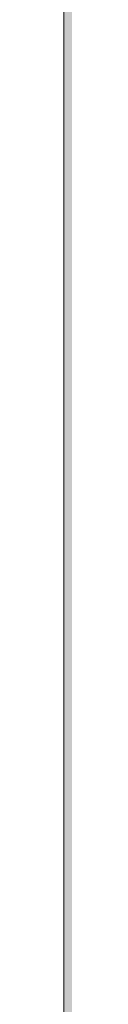
# Model space of a CAD drawing. Units: inches. Extents: x 459864 to 460310, y 324185 to 324787.
# Tile 34 of 112: x 460077.909 to 460077.909, y 324235.812 to 324241.994. Entities that reach past the tile are written whole.
import ezdxf

# ---------------------------------------------------------------- set-up
doc = ezdxf.new("R2010")
doc.units = ezdxf.units.IN
for name, color, linetype, lineweight in [('A-ANNO-DIMS', 2, 'Continuous', 18), ('L-HRDS', 9, 'Continuous', 18), ('L-SITE-PATT', 252, 'Continuous', 13)]:
    doc.layers.add(name, color=color, linetype=linetype, lineweight=lineweight)
doc.styles.get("Standard").update_dxf_attribs({"font": 'arial.ttf'})
doc.dimstyles.new('ISO-25', dxfattribs={"dimtxt": 6, "dimasz": 2.5, "dimexe": 1.25, "dimexo": 0.625, "dimtad": 1, "dimdec": 1, "dimlunit": 3, "dimtxsty": 'Standard', "dimcen": 2.5, "dimadec": 0, "dimazin": 0, "dimtfac": 1, "dimtdec": 1, "dimtmove": 0, "dimatfit": 3, "dimfxl": 1, "dimarcsym": 0})

# ---------------------------------------------------------------- blocks, each defined once
blk = doc.blocks.new('*D36')
at = {"layer": 'A-ANNO-DIMS', "color": 0, "lineweight": -2, "transparency": 16777216}
for p, q in [((460063.8613, 324228.4828), (460063.8613, 324226.0557)), ((460075.8757, 324228.4828), (460075.8757, 324226.0557)), ((460066.3613, 324227.3057), (460073.3757, 324227.3057)), ((460075.8757, 324227.3057), (460126.0214, 324227.3057))]:
    blk.add_line(p, q, dxfattribs=at)
at = {"layer": 'A-ANNO-DIMS', "color": 0, "transparency": 16777216}
for points in [[(460066.3613, 324227.7223), (460066.3613, 324226.889), (460063.8613, 324227.3057)], [(460073.3757, 324227.7223), (460073.3757, 324226.889), (460075.8757, 324227.3057)]]:
    blk.add_solid(points, dxfattribs=at)
at = {"layer": 'Defpoints', "color": 0, "transparency": 16777216}
for p in [(460063.8613, 324229.1078), (460075.8757, 324229.1078), (460075.8757, 324227.3057)]:
    blk.add_point(p, dxfattribs=at)
at = {"layer": 'A-ANNO-DIMS', "color": 0, "transparency": 16777216, "insert": (460102.1986, 324230.9941), "char_height": 6, "attachment_point": 5}
blk.add_mtext('PAVER 1\'-0"', dxfattribs=at)

msp = doc.modelspace()

# ---------------------------------------------------------------- hatches: boundary and pattern name
at = {"layer": 'L-SITE-PATT'}
h = msp.add_hatch(dxfattribs=at)
h.set_pattern_fill('DOTS', color=256)
h.paths.add_polyline_path([(460269.8036, 324283.4832), (460247.1149, 324283.4832), (460121.9293, 324283.4832), (460121.9293, 324252.473), (460117.4293, 324252.473), (460110.1236, 324252.473), (460110.1236, 324243.2865), (460080.8295, 324243.2865), (460080.8295, 324252.473), (460061.1149, 324252.473), (460061.1149, 324251.8824), (460077.9089, 324251.8824), (460077.9089, 324199.4832), (460080.8295, 324199.4832), (460080.8295, 324207.5532), (460110.1236, 324207.5532), (460110.1236, 324199.4832), (460110.8133, 324199.4832), (460262.1149, 324199.4832), (460269.8036, 324199.4832)], flags=17)
edge = h.paths.add_edge_path(flags=0)
edge.add_ellipse((460222.5903, 324263.8132), major_axis=(-8.4853, 8.4853), ratio=1, start_angle=405, end_angle=495, ccw=False)
edge.add_line((460214.8209, 324254.6599), (460214.8316, 324254.6659))
edge.add_ellipse((460222.5903, 324263.8132), major_axis=(-8.4853, 8.4853), ratio=1, start_angle=405, end_angle=495, ccw=False)
edge.add_line((460210.7589, 324261.7806), (460210.7676, 324261.7868))
edge.add_ellipse((460222.5903, 324263.8132), major_axis=(-8.4853, 8.4853), ratio=1, start_angle=405, end_angle=495, ccw=False)
edge.add_ellipse((460222.5903, 324263.8132), major_axis=(-8.4853, 8.4853), ratio=1, start_angle=392.75402, end_angle=405, ccw=False)
edge.add_ellipse((460222.5903, 324263.8132), major_axis=(-8.4853, 8.4853), ratio=1, start_angle=380.93472, end_angle=392.75402, ccw=False)
edge.add_line((460211.3371, 324267.985), (460211.3404, 324267.985))
edge.add_ellipse((460222.5903, 324263.8132), major_axis=(-8.4853, 8.4853), ratio=1, start_angle=380.93472, end_angle=392.75402, ccw=False)
edge.add_ellipse((460222.5903, 324263.8132), major_axis=(-8.4853, 8.4853), ratio=1, start_angle=347.90152, end_angle=380.93472, ccw=False)
edge.add_ellipse((460222.5903, 324263.8132), major_axis=(-8.4853, 8.4853), ratio=1, start_angle=327.06192, end_angle=347.90152, ccw=False)
edge.add_ellipse((460222.5903, 324263.8132), major_axis=(-8.4853, 8.4853), ratio=1, start_angle=278.32464, end_angle=327.06192, ccw=False)
edge.add_line((460225.1583, 324275.536), (460225.1577, 324275.5346))
edge.add_ellipse((460222.5903, 324263.8132), major_axis=(-8.4853, 8.4853), ratio=1, start_angle=278.32464, end_angle=327.06192, ccw=False)
edge.add_ellipse((460222.5903, 324263.8132), major_axis=(-8.4853, 8.4853), ratio=1, start_angle=260.64357, end_angle=278.32464, ccw=False)
edge.add_ellipse((460222.5903, 324263.8132), major_axis=(-8.4853, 8.4853), ratio=1, start_angle=225, end_angle=260.64357, ccw=False)
edge.add_line((460234.5088, 324265.2428), (460234.5015, 324265.2394))
edge.add_ellipse((460222.5903, 324263.8132), major_axis=(-8.4853, 8.4853), ratio=1, start_angle=225, end_angle=260.64357, ccw=False)
edge.add_ellipse((460222.5903, 324263.8132), major_axis=(-8.4853, 8.4853), ratio=1, start_angle=495, end_angle=585, ccw=False)
edge.add_line((460234.4367, 324261.8612), (460234.4238, 324261.8578))
edge.add_ellipse((460222.5903, 324263.8132), major_axis=(-8.4853, 8.4853), ratio=1, start_angle=495, end_angle=585, ccw=False)
edge.add_line((460227.9501, 324253.0672), (460227.9464, 324253.0831))
edge.add_ellipse((460222.5903, 324263.8132), major_axis=(-8.4853, 8.4853), ratio=1, start_angle=495, end_angle=585, ccw=False)
edge.add_line((460226.223, 324252.3693), (460226.211, 324252.3796))
edge.add_ellipse((460222.5903, 324263.8132), major_axis=(-8.4853, 8.4853), ratio=1, start_angle=495, end_angle=585, ccw=False)
h.paths.add_polyline_path([(460219.6515, 324254.3467), (460218.4613, 324253.545), (460218.2754, 324254.7893), (460219.6424, 324256.5418), (460219.6246, 324260.8476), (460216.1101, 324257.333), (460214.35, 324256.9781), (460215.4164, 324259.3557), (460212.5239, 324258.4958), (460213.1373, 324259.9298), (460218.5072, 324263.8132), (460222.5903, 324263.8132), (460222.5903, 324267.8067), (460218.1755, 324272.2123), (460219.026, 324274.639), (460222.5903, 324272.8111), (460222.5903, 324275.4233), (460223.0571, 324274.8249), (460222.6752, 324273.4922), (460225.9117, 324267.1346), (460219.6246, 324260.8476)], flags=0)
edge = h.paths.add_edge_path(flags=0)
edge.add_ellipse((460194.5758, 324264.0465), major_axis=(-8.4853, 8.4853), ratio=1, start_angle=495, end_angle=585, ccw=False)
edge.add_line((460199.9356, 324253.3005), (460199.9319, 324253.3164))
edge.add_ellipse((460194.5758, 324264.0465), major_axis=(-8.4853, 8.4853), ratio=1, start_angle=495, end_angle=585, ccw=False)
edge.add_line((460198.2084, 324252.6025), (460198.1965, 324252.6128))
edge.add_ellipse((460194.5758, 324264.0465), major_axis=(-8.4853, 8.4853), ratio=1, start_angle=495, end_angle=585, ccw=False)
edge.add_ellipse((460194.5758, 324264.0465), major_axis=(-8.4853, 8.4853), ratio=1, start_angle=405, end_angle=495, ccw=False)
edge.add_line((460186.8063, 324254.8932), (460186.8171, 324254.8992))
edge.add_ellipse((460194.5758, 324264.0465), major_axis=(-8.4853, 8.4853), ratio=1, start_angle=405, end_angle=495, ccw=False)
edge.add_line((460182.7444, 324262.0138), (460182.753, 324262.0201))
edge.add_ellipse((460194.5758, 324264.0465), major_axis=(-8.4853, 8.4853), ratio=1, start_angle=405, end_angle=495, ccw=False)
edge.add_ellipse((460194.5758, 324264.0465), major_axis=(-8.4853, 8.4853), ratio=1, start_angle=392.75402, end_angle=405, ccw=False)
edge.add_ellipse((460194.5758, 324264.0465), major_axis=(-8.4853, 8.4853), ratio=1, start_angle=380.93472, end_angle=392.75402, ccw=False)
edge.add_line((460183.3225, 324268.2183), (460183.3259, 324268.2183))
edge.add_ellipse((460194.5758, 324264.0465), major_axis=(-8.4853, 8.4853), ratio=1, start_angle=380.93472, end_angle=392.75402, ccw=False)
edge.add_ellipse((460194.5758, 324264.0465), major_axis=(-8.4853, 8.4853), ratio=1, start_angle=347.90152, end_angle=380.93472, ccw=False)
edge.add_ellipse((460194.5758, 324264.0465), major_axis=(-8.4853, 8.4853), ratio=1, start_angle=327.06192, end_angle=347.90152, ccw=False)
edge.add_ellipse((460194.5758, 324264.0465), major_axis=(-8.4853, 8.4853), ratio=1, start_angle=278.32464, end_angle=327.06192, ccw=False)
edge.add_line((460197.1437, 324275.7693), (460197.1432, 324275.7679))
edge.add_ellipse((460194.5758, 324264.0465), major_axis=(-8.4853, 8.4853), ratio=1, start_angle=278.32464, end_angle=327.06192, ccw=False)
edge.add_ellipse((460194.5758, 324264.0465), major_axis=(-8.4853, 8.4853), ratio=1, start_angle=260.64357, end_angle=278.32464, ccw=False)
edge.add_ellipse((460194.5758, 324264.0465), major_axis=(-8.4853, 8.4853), ratio=1, start_angle=225, end_angle=260.64357, ccw=False)
edge.add_line((460206.4943, 324265.4761), (460206.4869, 324265.4727))
edge.add_ellipse((460194.5758, 324264.0465), major_axis=(-8.4853, 8.4853), ratio=1, start_angle=225, end_angle=260.64357, ccw=False)
edge.add_ellipse((460194.5758, 324264.0465), major_axis=(-8.4853, 8.4853), ratio=1, start_angle=495, end_angle=585, ccw=False)
edge.add_line((460206.4221, 324262.0945), (460206.4092, 324262.0911))
h.paths.add_polyline_path([(460191.6101, 324261.0808), (460191.6369, 324254.5799), (460190.4468, 324253.7783), (460190.2609, 324255.0226), (460191.6279, 324256.775), (460191.6101, 324261.0808), (460188.0956, 324257.5663), (460186.3354, 324257.2113), (460187.4018, 324259.5889), (460184.5094, 324258.7291), (460185.1228, 324260.1631), (460190.4927, 324264.0465), (460194.5758, 324264.0465), (460194.5758, 324268.04), (460190.161, 324272.4456), (460191.0114, 324274.8722), (460194.5758, 324273.0444), (460194.5758, 324275.6566), (460195.0426, 324275.0582), (460194.6607, 324273.7255), (460197.8971, 324267.3679)], flags=0)
edge = h.paths.add_edge_path(flags=0)
edge.add_ellipse((460252.912, 324263.5776), major_axis=(-8.4853, 8.4853), ratio=1, start_angle=405, end_angle=495, ccw=False)
edge.add_line((460241.0806, 324261.5449), (460241.0892, 324261.5512))
edge.add_ellipse((460252.912, 324263.5776), major_axis=(-8.4853, 8.4853), ratio=1, start_angle=405, end_angle=495, ccw=False)
edge.add_ellipse((460252.912, 324263.5776), major_axis=(-8.4853, 8.4853), ratio=1, start_angle=392.75402, end_angle=405, ccw=False)
edge.add_ellipse((460252.912, 324263.5776), major_axis=(-8.4853, 8.4853), ratio=1, start_angle=380.93472, end_angle=392.75402, ccw=False)
edge.add_line((460241.6587, 324267.7494), (460241.6621, 324267.7494))
edge.add_ellipse((460252.912, 324263.5776), major_axis=(-8.4853, 8.4853), ratio=1, start_angle=380.93472, end_angle=392.75402, ccw=False)
edge.add_ellipse((460252.912, 324263.5776), major_axis=(-8.4853, 8.4853), ratio=1, start_angle=347.90152, end_angle=380.93472, ccw=False)
edge.add_ellipse((460252.912, 324263.5776), major_axis=(-8.4853, 8.4853), ratio=1, start_angle=327.06192, end_angle=347.90152, ccw=False)
edge.add_ellipse((460252.912, 324263.5776), major_axis=(-8.4853, 8.4853), ratio=1, start_angle=278.32464, end_angle=327.06192, ccw=False)
edge.add_line((460255.4799, 324275.3004), (460255.4794, 324275.299))
edge.add_ellipse((460252.912, 324263.5776), major_axis=(-8.4853, 8.4853), ratio=1, start_angle=278.32464, end_angle=327.06192, ccw=False)
edge.add_ellipse((460252.912, 324263.5776), major_axis=(-8.4853, 8.4853), ratio=1, start_angle=260.64357, end_angle=278.32464, ccw=False)
edge.add_ellipse((460252.912, 324263.5776), major_axis=(-8.4853, 8.4853), ratio=1, start_angle=225, end_angle=260.64357, ccw=False)
edge.add_line((460264.8305, 324265.0072), (460264.8231, 324265.0038))
edge.add_ellipse((460252.912, 324263.5776), major_axis=(-8.4853, 8.4853), ratio=1, start_angle=225, end_angle=260.64357, ccw=False)
edge.add_ellipse((460252.912, 324263.5776), major_axis=(-8.4853, 8.4853), ratio=1, start_angle=495, end_angle=585, ccw=False)
edge.add_line((460264.7583, 324261.6256), (460264.7454, 324261.6222))
edge.add_ellipse((460252.912, 324263.5776), major_axis=(-8.4853, 8.4853), ratio=1, start_angle=495, end_angle=585, ccw=False)
edge.add_line((460258.2718, 324252.8316), (460258.2681, 324252.8475))
edge.add_ellipse((460252.912, 324263.5776), major_axis=(-8.4853, 8.4853), ratio=1, start_angle=495, end_angle=585, ccw=False)
edge.add_line((460256.5446, 324252.1337), (460256.5327, 324252.1439))
edge.add_ellipse((460252.912, 324263.5776), major_axis=(-8.4853, 8.4853), ratio=1, start_angle=495, end_angle=585, ccw=False)
edge.add_ellipse((460252.912, 324263.5776), major_axis=(-8.4853, 8.4853), ratio=1, start_angle=405, end_angle=495, ccw=False)
edge.add_line((460245.1425, 324254.4243), (460245.1533, 324254.4303))
h.paths.add_polyline_path([(460244.6716, 324256.7425), (460245.738, 324259.1201), (460242.8456, 324258.2602), (460243.459, 324259.6942), (460248.8289, 324263.5776), (460252.912, 324263.5776), (460252.912, 324267.5711), (460248.4972, 324271.9767), (460249.3476, 324274.4034), (460252.912, 324272.5755), (460252.912, 324275.1877), (460253.3788, 324274.5893), (460252.9969, 324273.2566), (460256.2333, 324266.899), (460249.9463, 324260.612), (460249.9731, 324254.111), (460248.783, 324253.3094), (460248.5971, 324254.5537), (460249.9641, 324256.3062), (460249.9463, 324260.612), (460246.4318, 324257.0974)], flags=0)
edge = h.paths.add_edge_path(flags=0)
edge.add_ellipse((460167.4387, 324262.8328), major_axis=(-8.4853, 8.4853), ratio=1, start_angle=495, end_angle=585, ccw=False)
edge.add_line((460172.7985, 324252.0868), (460172.7948, 324252.1027))
edge.add_ellipse((460167.4387, 324262.8328), major_axis=(-8.4853, 8.4853), ratio=1, start_angle=495, end_angle=585, ccw=False)
edge.add_line((460171.0714, 324251.3888), (460171.0594, 324251.3991))
edge.add_ellipse((460167.4387, 324262.8328), major_axis=(-8.4853, 8.4853), ratio=1, start_angle=495, end_angle=585, ccw=False)
edge.add_ellipse((460167.4387, 324262.8328), major_axis=(-8.4853, 8.4853), ratio=1, start_angle=405, end_angle=495, ccw=False)
edge.add_line((460159.6693, 324253.6795), (460159.68, 324253.6855))
edge.add_ellipse((460167.4387, 324262.8328), major_axis=(-8.4853, 8.4853), ratio=1, start_angle=405, end_angle=495, ccw=False)
edge.add_line((460155.6073, 324260.8001), (460155.616, 324260.8064))
edge.add_ellipse((460167.4387, 324262.8328), major_axis=(-8.4853, 8.4853), ratio=1, start_angle=405, end_angle=495, ccw=False)
edge.add_ellipse((460167.4387, 324262.8328), major_axis=(-8.4853, 8.4853), ratio=1, start_angle=392.75402, end_angle=405, ccw=False)
edge.add_ellipse((460167.4387, 324262.8328), major_axis=(-8.4853, 8.4853), ratio=1, start_angle=380.93472, end_angle=392.75402, ccw=False)
edge.add_line((460156.1855, 324267.0046), (460156.1888, 324267.0046))
edge.add_ellipse((460167.4387, 324262.8328), major_axis=(-8.4853, 8.4853), ratio=1, start_angle=380.93472, end_angle=392.75402, ccw=False)
edge.add_ellipse((460167.4387, 324262.8328), major_axis=(-8.4853, 8.4853), ratio=1, start_angle=347.90152, end_angle=380.93472, ccw=False)
edge.add_ellipse((460167.4387, 324262.8328), major_axis=(-8.4853, 8.4853), ratio=1, start_angle=327.06192, end_angle=347.90152, ccw=False)
edge.add_ellipse((460167.4387, 324262.8328), major_axis=(-8.4853, 8.4853), ratio=1, start_angle=278.32464, end_angle=327.06192, ccw=False)
edge.add_line((460170.0067, 324274.5556), (460170.0061, 324274.5542))
edge.add_ellipse((460167.4387, 324262.8328), major_axis=(-8.4853, 8.4853), ratio=1, start_angle=278.32464, end_angle=327.06192, ccw=False)
edge.add_ellipse((460167.4387, 324262.8328), major_axis=(-8.4853, 8.4853), ratio=1, start_angle=260.64357, end_angle=278.32464, ccw=False)
edge.add_ellipse((460167.4387, 324262.8328), major_axis=(-8.4853, 8.4853), ratio=1, start_angle=225, end_angle=260.64357, ccw=False)
edge.add_line((460179.3572, 324264.2624), (460179.3499, 324264.259))
edge.add_ellipse((460167.4387, 324262.8328), major_axis=(-8.4853, 8.4853), ratio=1, start_angle=225, end_angle=260.64357, ccw=False)
edge.add_ellipse((460167.4387, 324262.8328), major_axis=(-8.4853, 8.4853), ratio=1, start_angle=495, end_angle=585, ccw=False)
edge.add_line((460179.2851, 324260.8808), (460179.2722, 324260.8774))
h.paths.add_polyline_path([(460164.473, 324259.8671), (460164.4998, 324253.3662), (460163.3097, 324252.5645), (460163.1238, 324253.8089), (460164.4908, 324255.5613), (460164.473, 324259.8671), (460160.9585, 324256.3526), (460159.1984, 324255.9976), (460160.2648, 324258.3752), (460157.3723, 324257.5154), (460157.9857, 324258.9494), (460163.3556, 324262.8328), (460167.4387, 324262.8328), (460167.4387, 324266.8263), (460163.0239, 324271.2319), (460163.8744, 324273.6585), (460167.4387, 324271.8307), (460167.4387, 324274.4429), (460167.9055, 324273.8445), (460167.5236, 324272.5118), (460170.7601, 324266.1542)], flags=0)
edge = h.paths.add_edge_path(flags=0)
edge.add_ellipse((460140.7581, 324262.3696), major_axis=(-8.4853, 8.4853), ratio=1, start_angle=495, end_angle=585, ccw=False)
edge.add_line((460146.1179, 324251.6235), (460146.1142, 324251.6395))
edge.add_ellipse((460140.7581, 324262.3696), major_axis=(-8.4853, 8.4853), ratio=1, start_angle=495, end_angle=585, ccw=False)
edge.add_line((460144.3908, 324250.9256), (460144.3788, 324250.9359))
edge.add_ellipse((460140.7581, 324262.3696), major_axis=(-8.4853, 8.4853), ratio=1, start_angle=495, end_angle=585, ccw=False)
edge.add_ellipse((460140.7581, 324262.3696), major_axis=(-8.4853, 8.4853), ratio=1, start_angle=405, end_angle=495, ccw=False)
edge.add_line((460132.9887, 324253.2162), (460132.9994, 324253.2223))
edge.add_ellipse((460140.7581, 324262.3696), major_axis=(-8.4853, 8.4853), ratio=1, start_angle=405, end_angle=495, ccw=False)
edge.add_line((460128.9267, 324260.3369), (460128.9354, 324260.3432))
edge.add_ellipse((460140.7581, 324262.3696), major_axis=(-8.4853, 8.4853), ratio=1, start_angle=405, end_angle=495, ccw=False)
edge.add_ellipse((460140.7581, 324262.3696), major_axis=(-8.4853, 8.4853), ratio=1, start_angle=392.75402, end_angle=405, ccw=False)
edge.add_ellipse((460140.7581, 324262.3696), major_axis=(-8.4853, 8.4853), ratio=1, start_angle=380.93472, end_angle=392.75402, ccw=False)
edge.add_line((460129.5049, 324266.5414), (460129.5082, 324266.5414))
edge.add_ellipse((460140.7581, 324262.3696), major_axis=(-8.4853, 8.4853), ratio=1, start_angle=380.93472, end_angle=392.75402, ccw=False)
edge.add_ellipse((460140.7581, 324262.3696), major_axis=(-8.4853, 8.4853), ratio=1, start_angle=347.90152, end_angle=380.93472, ccw=False)
edge.add_ellipse((460140.7581, 324262.3696), major_axis=(-8.4853, 8.4853), ratio=1, start_angle=327.06192, end_angle=347.90152, ccw=False)
edge.add_ellipse((460140.7581, 324262.3696), major_axis=(-8.4853, 8.4853), ratio=1, start_angle=278.32464, end_angle=327.06192, ccw=False)
edge.add_line((460143.3261, 324274.0923), (460143.3255, 324274.091))
edge.add_ellipse((460140.7581, 324262.3696), major_axis=(-8.4853, 8.4853), ratio=1, start_angle=278.32464, end_angle=327.06192, ccw=False)
edge.add_ellipse((460140.7581, 324262.3696), major_axis=(-8.4853, 8.4853), ratio=1, start_angle=260.64357, end_angle=278.32464, ccw=False)
edge.add_ellipse((460140.7581, 324262.3696), major_axis=(-8.4853, 8.4853), ratio=1, start_angle=225, end_angle=260.64357, ccw=False)
edge.add_line((460152.6766, 324263.7992), (460152.6692, 324263.7958))
edge.add_ellipse((460140.7581, 324262.3696), major_axis=(-8.4853, 8.4853), ratio=1, start_angle=225, end_angle=260.64357, ccw=False)
edge.add_ellipse((460140.7581, 324262.3696), major_axis=(-8.4853, 8.4853), ratio=1, start_angle=495, end_angle=585, ccw=False)
edge.add_line((460152.6045, 324260.4176), (460152.5916, 324260.4142))
h.paths.add_polyline_path([(460137.7924, 324259.4039), (460137.8192, 324252.903), (460136.6291, 324252.1013), (460136.4432, 324253.3457), (460137.8102, 324255.0981), (460137.7924, 324259.4039), (460134.2779, 324255.8894), (460132.5178, 324255.5344), (460133.5842, 324257.912), (460130.6917, 324257.0522), (460131.3051, 324258.4862), (460136.675, 324262.3696), (460140.7581, 324262.3696), (460140.7581, 324266.3631), (460136.3433, 324270.7687), (460137.1938, 324273.1953), (460140.7581, 324271.3675), (460140.7581, 324273.9797), (460141.2249, 324273.3813), (460140.843, 324272.0486), (460144.0795, 324265.691)], flags=0)
h.paths.add_polyline_path([(460110.1236, 324227.4139), (460080.8295, 324227.4139), (460080.8295, 324235.4839), (460110.1236, 324235.4839)], flags=16)
h.paths.add_polyline_path([(460110.1236, 324220.7966), (460110.1236, 324212.7267), (460080.8295, 324212.7267), (460080.8295, 324220.7966)], flags=16)
h.paths.add_polyline_path([(460269.8036, 324283.4832), (460247.1149, 324283.4832), (460121.9293, 324283.4832), (460121.9293, 324252.473), (460117.4293, 324252.473), (460110.1236, 324252.473), (460110.1236, 324243.2865), (460080.8295, 324243.2865), (460080.8295, 324252.473), (460061.1149, 324252.473), (460061.1149, 324251.8824), (460077.9089, 324251.8824), (460077.9089, 324199.4832), (460080.8295, 324199.4832), (460080.8295, 324207.5532), (460110.1236, 324207.5532), (460110.1236, 324199.4832), (460262.1149, 324199.4832), (460269.8036, 324199.4832)], flags=17)
h.paths.add_polyline_path([(460219.6515, 324254.3467), (460218.4613, 324253.545), (460218.2754, 324254.7893), (460219.6424, 324256.5418), (460219.6246, 324260.8476), (460216.1101, 324257.333), (460214.35, 324256.9781), (460215.4164, 324259.3557), (460212.5239, 324258.4958), (460213.1373, 324259.9298), (460218.5072, 324263.8132), (460222.5903, 324263.8132), (460220.1805, 324266.223), (460215.461, 324265.3076), (460211.8345, 324266.1366), (460216.2466, 324267.985), (460218.4185, 324267.985), (460222.5903, 324263.8132), (460222.5903, 324267.8067), (460218.1755, 324272.2123), (460219.026, 324274.639), (460222.5903, 324272.8111), (460222.5903, 324275.4233), (460223.0571, 324274.8249), (460222.6752, 324273.4922), (460225.9117, 324267.1346), (460222.5903, 324263.8132), (460231.3829, 324263.8132), (460228.4847, 324262.4878), (460224.4252, 324261.9783), (460228.6799, 324257.7236), (460228.9658, 324254.791), (460227.1418, 324256.5366), (460227.5421, 324254.8186), (460227.3333, 324253.6145), (460222.5903, 324259.9846), (460222.5903, 324255.4967), (460221.3774, 324256.5408), (460220.5758, 324261.7987), (460219.6246, 324260.8476)], flags=0)
h.paths.add_polyline_path([(460199.1272, 324256.7699), (460199.5275, 324255.0518), (460199.3188, 324253.8477), (460194.5758, 324260.2179), (460194.5758, 324255.7299), (460193.3629, 324256.7741), (460192.5613, 324262.032), (460191.6101, 324261.0808), (460191.6369, 324254.5799), (460190.4468, 324253.7783), (460190.2609, 324255.0226), (460191.6279, 324256.775), (460191.6101, 324261.0808), (460188.0956, 324257.5663), (460186.3354, 324257.2113), (460187.4018, 324259.5889), (460184.5094, 324258.7291), (460185.1228, 324260.1631), (460190.4927, 324264.0465), (460194.5758, 324264.0465), (460192.1659, 324266.4563), (460187.4464, 324265.5409), (460183.82, 324266.3698), (460188.2321, 324268.2183), (460190.404, 324268.2183), (460194.5758, 324264.0465), (460194.5758, 324268.04), (460190.161, 324272.4456), (460191.0114, 324274.8722), (460194.5758, 324273.0444), (460194.5758, 324275.6566), (460195.0426, 324275.0582), (460194.6607, 324273.7255), (460197.8971, 324267.3679), (460194.5758, 324264.0465), (460203.3683, 324264.0465), (460200.4702, 324262.7211), (460196.4107, 324262.2116), (460200.6654, 324257.9569), (460200.9513, 324255.0243)], flags=0)
h.paths.add_polyline_path([(460244.6716, 324256.7425), (460245.738, 324259.1201), (460242.8456, 324258.2602), (460243.459, 324259.6942), (460248.8289, 324263.5776), (460252.912, 324263.5776), (460250.5022, 324265.9874), (460245.7826, 324265.072), (460242.1562, 324265.9009), (460246.5683, 324267.7494), (460248.7402, 324267.7494), (460252.912, 324263.5776), (460252.912, 324267.5711), (460248.4972, 324271.9767), (460249.3476, 324274.4034), (460252.912, 324272.5755), (460252.912, 324275.1877), (460253.3788, 324274.5893), (460252.9969, 324273.2566), (460256.2333, 324266.899), (460252.912, 324263.5776), (460261.7045, 324263.5776), (460258.8064, 324262.2522), (460254.7469, 324261.7427), (460259.0016, 324257.488), (460259.2875, 324254.5554), (460257.4634, 324256.301), (460257.8637, 324254.583), (460257.655, 324253.3789), (460252.912, 324259.749), (460252.912, 324255.2611), (460251.6991, 324256.3052), (460250.8975, 324261.5631), (460249.9463, 324260.612), (460249.9731, 324254.111), (460248.783, 324253.3094), (460248.5971, 324254.5537), (460249.9641, 324256.3062), (460249.9463, 324260.612), (460246.4318, 324257.0974)], flags=0)
h.paths.add_polyline_path([(460173.5283, 324256.7432), (460173.8142, 324253.8106), (460171.9902, 324255.5562), (460172.3905, 324253.8381), (460172.1817, 324252.634), (460167.4387, 324259.0042), (460167.4387, 324254.5162), (460166.2258, 324255.5604), (460165.4242, 324260.8183), (460164.473, 324259.8671), (460164.4998, 324253.3662), (460163.3097, 324252.5645), (460163.1238, 324253.8089), (460164.4908, 324255.5613), (460164.473, 324259.8671), (460160.9585, 324256.3526), (460159.1984, 324255.9976), (460160.2648, 324258.3752), (460157.3723, 324257.5154), (460157.9857, 324258.9494), (460163.3556, 324262.8328), (460167.4387, 324262.8328), (460165.0289, 324265.2426), (460160.3094, 324264.3272), (460156.6829, 324265.1561), (460161.095, 324267.0046), (460163.2669, 324267.0046), (460167.4387, 324262.8328), (460167.4387, 324266.8263), (460163.0239, 324271.2319), (460163.8744, 324273.6585), (460167.4387, 324271.8307), (460167.4387, 324274.4429), (460167.9055, 324273.8445), (460167.5236, 324272.5118), (460170.7601, 324266.1542), (460167.4387, 324262.8328), (460176.2313, 324262.8328), (460173.3331, 324261.5074), (460169.2736, 324260.9979)], flags=0)
h.paths.add_polyline_path([(460146.8477, 324256.28), (460147.1336, 324253.3474), (460145.3096, 324255.093), (460145.7099, 324253.3749), (460145.5011, 324252.1708), (460140.7581, 324258.541), (460140.7581, 324254.053), (460139.5452, 324255.0972), (460138.7436, 324260.3551), (460137.7924, 324259.4039), (460137.8192, 324252.903), (460136.6291, 324252.1013), (460136.4432, 324253.3457), (460137.8102, 324255.0981), (460137.7924, 324259.4039), (460134.2779, 324255.8894), (460132.5178, 324255.5344), (460133.5842, 324257.912), (460130.6917, 324257.0522), (460131.3051, 324258.4862), (460136.675, 324262.3696), (460140.7581, 324262.3696), (460138.3483, 324264.7794), (460133.6288, 324263.864), (460130.0023, 324264.6929), (460134.4144, 324266.5414), (460136.5863, 324266.5414), (460140.7581, 324262.3696), (460140.7581, 324266.3631), (460136.3433, 324270.7687), (460137.1938, 324273.1953), (460140.7581, 324271.3675), (460140.7581, 324273.9797), (460141.2249, 324273.3813), (460140.843, 324272.0486), (460144.0795, 324265.691), (460140.7581, 324262.3696), (460149.5507, 324262.3696), (460146.6525, 324261.0442), (460142.593, 324260.5347)], flags=0)
edge = h.paths.add_edge_path()
edge.add_line((460269.8036, 324272.5491), (460260.8815, 324272.5491))
edge.add_ellipse((460252.912, 324263.5776), major_axis=(-8.4853, 8.4853), ratio=1, start_angle=260.64357, end_angle=273.38462, ccw=False)
edge.add_line((460262.2826, 324271.0921), (460262.2606, 324271.0911))
edge.add_ellipse((460252.912, 324263.5776), major_axis=(-8.4853, 8.4853), ratio=1, start_angle=260.64357, end_angle=273.38462, ccw=False)
edge.add_ellipse((460252.912, 324263.5776), major_axis=(-8.4853, 8.4853), ratio=1, start_angle=225, end_angle=260.64357, ccw=False)
edge.add_line((460263.6086, 324269.0633), (460263.5717, 324269.0583))
edge.add_ellipse((460252.912, 324263.5776), major_axis=(-8.4853, 8.4853), ratio=1, start_angle=225, end_angle=260.64357, ccw=False)
edge.add_line((460264.6155, 324266.3055), (460264.5854, 324266.3052))
edge.add_ellipse((460252.912, 324263.5776), major_axis=(-8.4853, 8.4853), ratio=1, start_angle=225, end_angle=260.64357, ccw=False)
edge.add_line((460264.8305, 324265.0072), (460264.8231, 324265.0038))
edge.add_ellipse((460252.912, 324263.5776), major_axis=(-8.4853, 8.4853), ratio=1, start_angle=225, end_angle=260.64357, ccw=False)
edge.add_ellipse((460252.912, 324263.5776), major_axis=(-8.4853, 8.4853), ratio=1, start_angle=495, end_angle=585, ccw=False)
edge.add_line((460264.7583, 324261.6256), (460264.7454, 324261.6222))
edge.add_ellipse((460252.912, 324263.5776), major_axis=(-8.4853, 8.4853), ratio=1, start_angle=495, end_angle=585, ccw=False)
edge.add_line((460263.4422, 324257.739), (460263.3893, 324257.7792))
edge.add_ellipse((460252.912, 324263.5776), major_axis=(-8.4853, 8.4853), ratio=1, start_angle=495, end_angle=585, ccw=False)
edge.add_line((460258.1281, 324252.7435), (460258.1019, 324252.7787))
edge.add_ellipse((460252.912, 324263.5776), major_axis=(-8.4853, 8.4853), ratio=1, start_angle=495, end_angle=585, ccw=False)
edge.add_line((460256.5446, 324252.1337), (460256.5327, 324252.1439))
edge.add_ellipse((460252.912, 324263.5776), major_axis=(-8.4853, 8.4853), ratio=1, start_angle=495, end_angle=585, ccw=False)
edge.add_ellipse((460252.912, 324263.5776), major_axis=(-8.4853, 8.4853), ratio=1, start_angle=405, end_angle=495, ccw=False)
edge.add_line((460250.594, 324251.7804), (460250.6047, 324251.8198))
edge.add_ellipse((460252.912, 324263.5776), major_axis=(-8.4853, 8.4853), ratio=1, start_angle=405, end_angle=495, ccw=False)
edge.add_line((460245.1425, 324254.4243), (460245.1533, 324254.4303))
edge.add_ellipse((460252.912, 324263.5776), major_axis=(-8.4853, 8.4853), ratio=1, start_angle=405, end_angle=495, ccw=False)
edge.add_line((460243.5246, 324256.059), (460243.5603, 324256.0914))
edge.add_ellipse((460252.912, 324263.5776), major_axis=(-8.4853, 8.4853), ratio=1, start_angle=405, end_angle=495, ccw=False)
edge.add_line((460241.4401, 324259.8927), (460241.5224, 324259.8959))
edge.add_ellipse((460252.912, 324263.5776), major_axis=(-8.4853, 8.4853), ratio=1, start_angle=405, end_angle=495, ccw=False)
edge.add_line((460241.0806, 324261.5449), (460241.0892, 324261.5512))
edge.add_ellipse((460252.912, 324263.5776), major_axis=(-8.4853, 8.4853), ratio=1, start_angle=405, end_angle=495, ccw=False)
edge.add_ellipse((460252.912, 324263.5776), major_axis=(-8.4853, 8.4853), ratio=1, start_angle=392.75402, end_angle=405, ccw=False)
edge.add_line((460241.0503, 324265.4376), (460241.0626, 324265.4428))
edge.add_ellipse((460252.912, 324263.5776), major_axis=(-8.4853, 8.4853), ratio=1, start_angle=392.75402, end_angle=405, ccw=False)
edge.add_ellipse((460252.912, 324263.5776), major_axis=(-8.4853, 8.4853), ratio=1, start_angle=380.93472, end_angle=392.75402, ccw=False)
edge.add_line((460241.4519, 324267.1764), (460241.469, 324267.171))
edge.add_ellipse((460252.912, 324263.5776), major_axis=(-8.4853, 8.4853), ratio=1, start_angle=380.93472, end_angle=392.75402, ccw=False)
edge.add_line((460241.6587, 324267.7494), (460241.6621, 324267.7494))
edge.add_ellipse((460252.912, 324263.5776), major_axis=(-8.4853, 8.4853), ratio=1, start_angle=380.93472, end_angle=392.75402, ccw=False)
edge.add_ellipse((460252.912, 324263.5776), major_axis=(-8.4853, 8.4853), ratio=1, start_angle=356.61538, end_angle=380.93472, ccw=False)
edge.add_line((460244.8803, 324272.4877), (460244.7127, 324272.5491))
edge.add_line((460244.7127, 324272.5491), (460230.8174, 324272.5491))
edge.add_ellipse((460222.5903, 324263.8132), major_axis=(-8.4853, 8.4853), ratio=1, start_angle=260.64357, end_angle=271.71777, ccw=False)
edge.add_ellipse((460222.5903, 324263.8132), major_axis=(-8.4853, 8.4853), ratio=1, start_angle=225, end_angle=260.64357, ccw=False)
edge.add_line((460233.2869, 324269.2989), (460233.25, 324269.2939))
edge.add_ellipse((460222.5903, 324263.8132), major_axis=(-8.4853, 8.4853), ratio=1, start_angle=225, end_angle=260.64357, ccw=False)
edge.add_line((460234.2938, 324266.5412), (460234.2637, 324266.5408))
edge.add_ellipse((460222.5903, 324263.8132), major_axis=(-8.4853, 8.4853), ratio=1, start_angle=225, end_angle=260.64357, ccw=False)
edge.add_line((460234.5088, 324265.2428), (460234.5015, 324265.2394))
edge.add_ellipse((460222.5903, 324263.8132), major_axis=(-8.4853, 8.4853), ratio=1, start_angle=225, end_angle=260.64357, ccw=False)
edge.add_ellipse((460222.5903, 324263.8132), major_axis=(-8.4853, 8.4853), ratio=1, start_angle=495, end_angle=585, ccw=False)
edge.add_line((460234.4367, 324261.8612), (460234.4238, 324261.8578))
edge.add_ellipse((460222.5903, 324263.8132), major_axis=(-8.4853, 8.4853), ratio=1, start_angle=495, end_angle=585, ccw=False)
edge.add_line((460233.1205, 324257.9746), (460233.0676, 324258.0149))
edge.add_ellipse((460222.5903, 324263.8132), major_axis=(-8.4853, 8.4853), ratio=1, start_angle=495, end_angle=585, ccw=False)
edge.add_line((460227.8064, 324252.9791), (460227.7802, 324253.0143))
edge.add_ellipse((460222.5903, 324263.8132), major_axis=(-8.4853, 8.4853), ratio=1, start_angle=495, end_angle=585, ccw=False)
edge.add_line((460226.223, 324252.3693), (460226.211, 324252.3796))
edge.add_ellipse((460222.5903, 324263.8132), major_axis=(-8.4853, 8.4853), ratio=1, start_angle=495, end_angle=585, ccw=False)
edge.add_ellipse((460222.5903, 324263.8132), major_axis=(-8.4853, 8.4853), ratio=1, start_angle=405, end_angle=495, ccw=False)
edge.add_line((460220.2723, 324252.016), (460220.283, 324252.0554))
edge.add_ellipse((460222.5903, 324263.8132), major_axis=(-8.4853, 8.4853), ratio=1, start_angle=405, end_angle=495, ccw=False)
edge.add_line((460214.8209, 324254.6599), (460214.8316, 324254.6659))
edge.add_ellipse((460222.5903, 324263.8132), major_axis=(-8.4853, 8.4853), ratio=1, start_angle=405, end_angle=495, ccw=False)
edge.add_line((460213.2029, 324256.2946), (460213.2387, 324256.327))
edge.add_ellipse((460222.5903, 324263.8132), major_axis=(-8.4853, 8.4853), ratio=1, start_angle=405, end_angle=495, ccw=False)
edge.add_line((460211.1184, 324260.1283), (460211.2008, 324260.1315))
edge.add_ellipse((460222.5903, 324263.8132), major_axis=(-8.4853, 8.4853), ratio=1, start_angle=405, end_angle=495, ccw=False)
edge.add_line((460210.7589, 324261.7806), (460210.7676, 324261.7868))
edge.add_ellipse((460222.5903, 324263.8132), major_axis=(-8.4853, 8.4853), ratio=1, start_angle=405, end_angle=495, ccw=False)
edge.add_ellipse((460222.5903, 324263.8132), major_axis=(-8.4853, 8.4853), ratio=1, start_angle=392.75402, end_angle=405, ccw=False)
edge.add_line((460210.7286, 324265.6732), (460210.7409, 324265.6784))
edge.add_ellipse((460222.5903, 324263.8132), major_axis=(-8.4853, 8.4853), ratio=1, start_angle=392.75402, end_angle=405, ccw=False)
edge.add_ellipse((460222.5903, 324263.8132), major_axis=(-8.4853, 8.4853), ratio=1, start_angle=380.93472, end_angle=392.75402, ccw=False)
edge.add_line((460211.1302, 324267.412), (460211.1474, 324267.4066))
edge.add_ellipse((460222.5903, 324263.8132), major_axis=(-8.4853, 8.4853), ratio=1, start_angle=380.93472, end_angle=392.75402, ccw=False)
edge.add_line((460211.3371, 324267.985), (460211.3404, 324267.985))
edge.add_ellipse((460222.5903, 324263.8132), major_axis=(-8.4853, 8.4853), ratio=1, start_angle=380.93472, end_angle=392.75402, ccw=False)
edge.add_ellipse((460222.5903, 324263.8132), major_axis=(-8.4853, 8.4853), ratio=1, start_angle=358.28223, end_angle=380.93472, ccw=False)
edge.add_line((460213.7045, 324271.9018), (460213.709, 324271.869))
edge.add_ellipse((460222.5903, 324263.8132), major_axis=(-8.4853, 8.4853), ratio=1, start_angle=358.28223, end_angle=380.93472, ccw=False)
edge.add_line((460214.3632, 324272.5491), (460203.0783, 324272.5491))
edge.add_line((460203.0783, 324272.5491), (460203.0603, 324272.5311))
edge.add_ellipse((460194.5758, 324264.0465), major_axis=(-8.4853, 8.4853), ratio=1, start_angle=260.64357, end_angle=270.11679, ccw=False)
edge.add_line((460203.9566, 324271.5615), (460203.9209, 324271.5598))
edge.add_ellipse((460194.5758, 324264.0465), major_axis=(-8.4853, 8.4853), ratio=1, start_angle=260.64357, end_angle=270.11679, ccw=False)
edge.add_ellipse((460194.5758, 324264.0465), major_axis=(-8.4853, 8.4853), ratio=1, start_angle=225, end_angle=260.64357, ccw=False)
edge.add_line((460205.2724, 324269.5322), (460205.2354, 324269.5272))
edge.add_ellipse((460194.5758, 324264.0465), major_axis=(-8.4853, 8.4853), ratio=1, start_angle=225, end_angle=260.64357, ccw=False)
edge.add_line((460206.2793, 324266.7744), (460206.2492, 324266.7741))
edge.add_ellipse((460194.5758, 324264.0465), major_axis=(-8.4853, 8.4853), ratio=1, start_angle=225, end_angle=260.64357, ccw=False)
edge.add_line((460206.4943, 324265.4761), (460206.4869, 324265.4727))
edge.add_ellipse((460194.5758, 324264.0465), major_axis=(-8.4853, 8.4853), ratio=1, start_angle=225, end_angle=260.64357, ccw=False)
edge.add_ellipse((460194.5758, 324264.0465), major_axis=(-8.4853, 8.4853), ratio=1, start_angle=495, end_angle=585, ccw=False)
edge.add_line((460206.4221, 324262.0945), (460206.4092, 324262.0911))
edge.add_ellipse((460194.5758, 324264.0465), major_axis=(-8.4853, 8.4853), ratio=1, start_angle=495, end_angle=585, ccw=False)
edge.add_line((460205.106, 324258.2079), (460205.0531, 324258.2481))
edge.add_ellipse((460194.5758, 324264.0465), major_axis=(-8.4853, 8.4853), ratio=1, start_angle=495, end_angle=585, ccw=False)
edge.add_line((460199.7919, 324253.2124), (460199.7657, 324253.2476))
edge.add_ellipse((460194.5758, 324264.0465), major_axis=(-8.4853, 8.4853), ratio=1, start_angle=495, end_angle=585, ccw=False)
edge.add_line((460198.2084, 324252.6025), (460198.1965, 324252.6128))
edge.add_ellipse((460194.5758, 324264.0465), major_axis=(-8.4853, 8.4853), ratio=1, start_angle=495, end_angle=585, ccw=False)
edge.add_ellipse((460194.5758, 324264.0465), major_axis=(-8.4853, 8.4853), ratio=1, start_angle=405, end_angle=495, ccw=False)
edge.add_line((460192.2578, 324252.2493), (460192.2684, 324252.2887))
edge.add_ellipse((460194.5758, 324264.0465), major_axis=(-8.4853, 8.4853), ratio=1, start_angle=405, end_angle=495, ccw=False)
edge.add_line((460186.8063, 324254.8932), (460186.8171, 324254.8992))
edge.add_ellipse((460194.5758, 324264.0465), major_axis=(-8.4853, 8.4853), ratio=1, start_angle=405, end_angle=495, ccw=False)
edge.add_line((460185.1884, 324256.5279), (460185.2241, 324256.5602))
edge.add_ellipse((460194.5758, 324264.0465), major_axis=(-8.4853, 8.4853), ratio=1, start_angle=405, end_angle=495, ccw=False)
edge.add_line((460183.1039, 324260.3616), (460183.1862, 324260.3648))
edge.add_ellipse((460194.5758, 324264.0465), major_axis=(-8.4853, 8.4853), ratio=1, start_angle=405, end_angle=495, ccw=False)
edge.add_line((460182.7444, 324262.0138), (460182.753, 324262.0201))
edge.add_ellipse((460194.5758, 324264.0465), major_axis=(-8.4853, 8.4853), ratio=1, start_angle=405, end_angle=495, ccw=False)
edge.add_ellipse((460194.5758, 324264.0465), major_axis=(-8.4853, 8.4853), ratio=1, start_angle=392.75402, end_angle=405, ccw=False)
edge.add_line((460182.7141, 324265.9065), (460182.7264, 324265.9116))
edge.add_ellipse((460194.5758, 324264.0465), major_axis=(-8.4853, 8.4853), ratio=1, start_angle=392.75402, end_angle=405, ccw=False)
edge.add_ellipse((460194.5758, 324264.0465), major_axis=(-8.4853, 8.4853), ratio=1, start_angle=380.93472, end_angle=392.75402, ccw=False)
edge.add_line((460183.1157, 324267.6453), (460183.1328, 324267.6399))
edge.add_ellipse((460194.5758, 324264.0465), major_axis=(-8.4853, 8.4853), ratio=1, start_angle=380.93472, end_angle=392.75402, ccw=False)
edge.add_line((460183.3225, 324268.2183), (460183.3259, 324268.2183))
edge.add_ellipse((460194.5758, 324264.0465), major_axis=(-8.4853, 8.4853), ratio=1, start_angle=380.93472, end_angle=392.75402, ccw=False)
edge.add_ellipse((460194.5758, 324264.0465), major_axis=(-8.4853, 8.4853), ratio=1, start_angle=359.88321, end_angle=380.93472, ccw=False)
edge.add_line((460184.4914, 324270.6108), (460184.5531, 324270.6108))
edge.add_ellipse((460194.5758, 324264.0465), major_axis=(-8.4853, 8.4853), ratio=1, start_angle=359.88321, end_angle=380.93472, ccw=False)
edge.add_line((460185.3458, 324271.7602), (460185.3786, 324271.728))
edge.add_ellipse((460194.5758, 324264.0465), major_axis=(-8.4853, 8.4853), ratio=1, start_angle=359.88321, end_angle=380.93472, ccw=False)
edge.add_line((460185.6967, 324272.0862), (460185.633, 324272.5491))
edge.add_line((460185.633, 324272.5491), (460174.6834, 324272.5491))
edge.add_line((460174.6834, 324272.5491), (460174.6061, 324272.4572))
edge.add_ellipse((460167.4387, 324262.8328), major_axis=(-8.4853, 8.4853), ratio=1, start_angle=260.64357, end_angle=278.32464, ccw=False)
edge.add_ellipse((460167.4387, 324262.8328), major_axis=(-8.4853, 8.4853), ratio=1, start_angle=225, end_angle=260.64357, ccw=False)
edge.add_line((460178.1353, 324268.3185), (460178.0984, 324268.3135))
edge.add_ellipse((460167.4387, 324262.8328), major_axis=(-8.4853, 8.4853), ratio=1, start_angle=225, end_angle=260.64357, ccw=False)
edge.add_line((460179.1422, 324265.5607), (460179.1121, 324265.5604))
edge.add_ellipse((460167.4387, 324262.8328), major_axis=(-8.4853, 8.4853), ratio=1, start_angle=225, end_angle=260.64357, ccw=False)
edge.add_line((460179.3572, 324264.2624), (460179.3499, 324264.259))
edge.add_ellipse((460167.4387, 324262.8328), major_axis=(-8.4853, 8.4853), ratio=1, start_angle=225, end_angle=260.64357, ccw=False)
edge.add_ellipse((460167.4387, 324262.8328), major_axis=(-8.4853, 8.4853), ratio=1, start_angle=495, end_angle=585, ccw=False)
edge.add_line((460179.2851, 324260.8808), (460179.2722, 324260.8774))
edge.add_ellipse((460167.4387, 324262.8328), major_axis=(-8.4853, 8.4853), ratio=1, start_angle=495, end_angle=585, ccw=False)
edge.add_line((460177.9689, 324256.9942), (460177.916, 324257.0344))
edge.add_ellipse((460167.4387, 324262.8328), major_axis=(-8.4853, 8.4853), ratio=1, start_angle=495, end_angle=585, ccw=False)
edge.add_line((460172.6548, 324251.9987), (460172.6286, 324252.0339))
edge.add_ellipse((460167.4387, 324262.8328), major_axis=(-8.4853, 8.4853), ratio=1, start_angle=495, end_angle=585, ccw=False)
edge.add_line((460171.0714, 324251.3888), (460171.0594, 324251.3991))
edge.add_ellipse((460167.4387, 324262.8328), major_axis=(-8.4853, 8.4853), ratio=1, start_angle=495, end_angle=585, ccw=False)
edge.add_ellipse((460167.4387, 324262.8328), major_axis=(-8.4853, 8.4853), ratio=1, start_angle=405, end_angle=495, ccw=False)
edge.add_line((460165.1207, 324251.0356), (460165.1314, 324251.075))
edge.add_ellipse((460167.4387, 324262.8328), major_axis=(-8.4853, 8.4853), ratio=1, start_angle=405, end_angle=495, ccw=False)
edge.add_line((460159.6693, 324253.6795), (460159.68, 324253.6855))
edge.add_ellipse((460167.4387, 324262.8328), major_axis=(-8.4853, 8.4853), ratio=1, start_angle=405, end_angle=495, ccw=False)
edge.add_line((460158.0513, 324255.3142), (460158.0871, 324255.3465))
edge.add_ellipse((460167.4387, 324262.8328), major_axis=(-8.4853, 8.4853), ratio=1, start_angle=405, end_angle=495, ccw=False)
edge.add_line((460155.9668, 324259.1479), (460156.0492, 324259.1511))
edge.add_ellipse((460167.4387, 324262.8328), major_axis=(-8.4853, 8.4853), ratio=1, start_angle=405, end_angle=495, ccw=False)
edge.add_line((460155.6073, 324260.8001), (460155.616, 324260.8064))
edge.add_ellipse((460167.4387, 324262.8328), major_axis=(-8.4853, 8.4853), ratio=1, start_angle=405, end_angle=495, ccw=False)
edge.add_ellipse((460167.4387, 324262.8328), major_axis=(-8.4853, 8.4853), ratio=1, start_angle=392.75402, end_angle=405, ccw=False)
edge.add_line((460155.577, 324264.6928), (460155.5893, 324264.6979))
edge.add_ellipse((460167.4387, 324262.8328), major_axis=(-8.4853, 8.4853), ratio=1, start_angle=392.75402, end_angle=405, ccw=False)
edge.add_ellipse((460167.4387, 324262.8328), major_axis=(-8.4853, 8.4853), ratio=1, start_angle=380.93472, end_angle=392.75402, ccw=False)
edge.add_line((460155.9786, 324266.4316), (460155.9958, 324266.4262))
edge.add_ellipse((460167.4387, 324262.8328), major_axis=(-8.4853, 8.4853), ratio=1, start_angle=380.93472, end_angle=392.75402, ccw=False)
edge.add_line((460156.1855, 324267.0046), (460156.1888, 324267.0046))
edge.add_ellipse((460167.4387, 324262.8328), major_axis=(-8.4853, 8.4853), ratio=1, start_angle=380.93472, end_angle=392.75402, ccw=False)
edge.add_ellipse((460167.4387, 324262.8328), major_axis=(-8.4853, 8.4853), ratio=1, start_angle=350.93449, end_angle=380.93472, ccw=False)
edge.add_line((460157.3633, 324269.3971), (460157.4144, 324269.3971))
edge.add_ellipse((460167.4387, 324262.8328), major_axis=(-8.4853, 8.4853), ratio=1, start_angle=350.93449, end_angle=380.93472, ccw=False)
edge.add_line((460158.2205, 324270.535), (460158.2365, 324270.5193))
edge.add_ellipse((460167.4387, 324262.8328), major_axis=(-8.4853, 8.4853), ratio=1, start_angle=350.93449, end_angle=380.93472, ccw=False)
edge.add_line((460159.3794, 324271.7529), (460159.4193, 324271.7383))
edge.add_ellipse((460167.4387, 324262.8328), major_axis=(-8.4853, 8.4853), ratio=1, start_angle=350.93449, end_angle=380.93472, ccw=False)
edge.add_line((460160.3964, 324272.5491), (460147.1125, 324272.5491))
edge.add_ellipse((460140.7581, 324262.3696), major_axis=(-8.4853, 8.4853), ratio=1, start_angle=278.32464, end_angle=283.02607, ccw=False)
edge.add_ellipse((460140.7581, 324262.3696), major_axis=(-8.4853, 8.4853), ratio=1, start_angle=260.64357, end_angle=278.32464, ccw=False)
edge.add_ellipse((460140.7581, 324262.3696), major_axis=(-8.4853, 8.4853), ratio=1, start_angle=225, end_angle=260.64357, ccw=False)
edge.add_line((460151.4547, 324267.8553), (460151.4178, 324267.8503))
edge.add_ellipse((460140.7581, 324262.3696), major_axis=(-8.4853, 8.4853), ratio=1, start_angle=225, end_angle=260.64357, ccw=False)
edge.add_line((460152.4616, 324265.0975), (460152.4315, 324265.0972))
edge.add_ellipse((460140.7581, 324262.3696), major_axis=(-8.4853, 8.4853), ratio=1, start_angle=225, end_angle=260.64357, ccw=False)
edge.add_line((460152.6766, 324263.7992), (460152.6692, 324263.7958))
edge.add_ellipse((460140.7581, 324262.3696), major_axis=(-8.4853, 8.4853), ratio=1, start_angle=225, end_angle=260.64357, ccw=False)
edge.add_ellipse((460140.7581, 324262.3696), major_axis=(-8.4853, 8.4853), ratio=1, start_angle=495, end_angle=585, ccw=False)
edge.add_line((460152.6045, 324260.4176), (460152.5916, 324260.4142))
edge.add_ellipse((460140.7581, 324262.3696), major_axis=(-8.4853, 8.4853), ratio=1, start_angle=495, end_angle=585, ccw=False)
edge.add_line((460151.2883, 324256.531), (460151.2354, 324256.5712))
edge.add_ellipse((460140.7581, 324262.3696), major_axis=(-8.4853, 8.4853), ratio=1, start_angle=495, end_angle=585, ccw=False)
edge.add_line((460145.9742, 324251.5355), (460145.948, 324251.5707))
edge.add_ellipse((460140.7581, 324262.3696), major_axis=(-8.4853, 8.4853), ratio=1, start_angle=495, end_angle=585, ccw=False)
edge.add_line((460144.3908, 324250.9256), (460144.3788, 324250.9359))
edge.add_ellipse((460140.7581, 324262.3696), major_axis=(-8.4853, 8.4853), ratio=1, start_angle=495, end_angle=585, ccw=False)
edge.add_ellipse((460140.7581, 324262.3696), major_axis=(-8.4853, 8.4853), ratio=1, start_angle=405, end_angle=495, ccw=False)
edge.add_line((460138.4401, 324250.5724), (460138.4508, 324250.6118))
edge.add_ellipse((460140.7581, 324262.3696), major_axis=(-8.4853, 8.4853), ratio=1, start_angle=405, end_angle=495, ccw=False)
edge.add_line((460132.9887, 324253.2162), (460132.9994, 324253.2223))
edge.add_ellipse((460140.7581, 324262.3696), major_axis=(-8.4853, 8.4853), ratio=1, start_angle=405, end_angle=495, ccw=False)
edge.add_line((460131.3707, 324254.851), (460131.4065, 324254.8833))
edge.add_ellipse((460140.7581, 324262.3696), major_axis=(-8.4853, 8.4853), ratio=1, start_angle=405, end_angle=495, ccw=False)
edge.add_line((460129.2862, 324258.6847), (460129.3686, 324258.6878))
edge.add_ellipse((460140.7581, 324262.3696), major_axis=(-8.4853, 8.4853), ratio=1, start_angle=405, end_angle=495, ccw=False)
edge.add_line((460128.9267, 324260.3369), (460128.9354, 324260.3432))
edge.add_ellipse((460140.7581, 324262.3696), major_axis=(-8.4853, 8.4853), ratio=1, start_angle=405, end_angle=495, ccw=False)
edge.add_ellipse((460140.7581, 324262.3696), major_axis=(-8.4853, 8.4853), ratio=1, start_angle=392.75402, end_angle=405, ccw=False)
edge.add_line((460128.8964, 324264.2296), (460128.9087, 324264.2347))
edge.add_ellipse((460140.7581, 324262.3696), major_axis=(-8.4853, 8.4853), ratio=1, start_angle=392.75402, end_angle=405, ccw=False)
edge.add_ellipse((460140.7581, 324262.3696), major_axis=(-8.4853, 8.4853), ratio=1, start_angle=380.93472, end_angle=392.75402, ccw=False)
edge.add_line((460129.298, 324265.9684), (460129.3152, 324265.963))
edge.add_ellipse((460140.7581, 324262.3696), major_axis=(-8.4853, 8.4853), ratio=1, start_angle=380.93472, end_angle=392.75402, ccw=False)
edge.add_line((460129.5049, 324266.5414), (460129.5082, 324266.5414))
edge.add_ellipse((460140.7581, 324262.3696), major_axis=(-8.4853, 8.4853), ratio=1, start_angle=380.93472, end_angle=392.75402, ccw=False)
edge.add_ellipse((460140.7581, 324262.3696), major_axis=(-8.4853, 8.4853), ratio=1, start_angle=347.90152, end_angle=380.93472, ccw=False)
edge.add_line((460130.6969, 324268.9339), (460130.7268, 324268.9339))
edge.add_ellipse((460140.7581, 324262.3696), major_axis=(-8.4853, 8.4853), ratio=1, start_angle=347.90152, end_angle=380.93472, ccw=False)
edge.add_line((460131.8693, 324270.4804), (460131.8786, 324270.4126))
edge.add_ellipse((460140.7581, 324262.3696), major_axis=(-8.4853, 8.4853), ratio=1, start_angle=347.90152, end_angle=380.93472, ccw=False)
edge.add_line((460132.7341, 324271.2768), (460132.7054, 324271.2873))
edge.add_ellipse((460140.7581, 324262.3696), major_axis=(-8.4853, 8.4853), ratio=1, start_angle=347.90152, end_angle=380.93472, ccw=False)
edge.add_line((460134.2397, 324272.4449), (460134.2035, 324272.5491))
edge.add_line((460134.2035, 324272.5491), (460121.9293, 324272.5491))
edge.add_line((460121.9293, 324272.5491), (460121.9293, 324252.473))
edge.add_line((460121.9293, 324252.473), (460117.4293, 324252.473))
edge.add_line((460117.4293, 324252.473), (460110.1236, 324252.473))
edge.add_line((460110.1236, 324252.473), (460110.1236, 324243.2865))
edge.add_line((460110.1236, 324243.2865), (460080.8295, 324243.2865))
edge.add_line((460080.8295, 324243.2865), (460080.8295, 324252.473))
edge.add_line((460080.8295, 324252.473), (460061.1149, 324252.473))
edge.add_line((460061.1149, 324252.473), (460061.1149, 324251.8824))
edge.add_line((460061.1149, 324251.8824), (460077.9089, 324251.8824))
edge.add_line((460077.9089, 324251.8824), (460077.9089, 324199.4832))
edge.add_line((460077.9089, 324199.4832), (460080.8295, 324199.4832))
edge.add_line((460080.8295, 324199.4832), (460080.8295, 324207.5532))
edge.add_line((460080.8295, 324207.5532), (460110.1236, 324207.5532))
edge.add_line((460110.1236, 324207.5532), (460110.1236, 324199.4832))
edge.add_line((460110.1236, 324199.4832), (460110.8133, 324199.4832))
edge.add_line((460110.8133, 324199.4832), (460262.1149, 324199.4832))
edge.add_line((460262.1149, 324199.4832), (460269.8036, 324199.4832))
edge.add_line((460269.8036, 324199.4832), (460269.8036, 324272.5491))
h = msp.add_hatch(dxfattribs=at)
h.set_pattern_fill('DOTS', color=256)
h.paths.add_polyline_path([(460077.9089, 324250.7795), (460061.1149, 324250.7795), (460061.1149, 324235.4832), (460061.1149, 324199.4832), (460077.9089, 324199.4832)])

# ---------------------------------------------------------------- linework, layer by layer
at = {"layer": 'L-HRDS'}
msp.add_line((460077.9089, 324251.8824), (460077.9089, 324199.4832), dxfattribs=at)

# ---------------------------------------------------------------- dimensions: what is measured, and where the dimension line sits
at = {"layer": 'A-ANNO-DIMS'}
dim = msp.add_linear_dim(base=(460075.8757, 324227.3057), p1=(460063.8613, 324229.1078), p2=(460075.8757, 324229.1078), text='PAVER <>', dimstyle='ISO-25', override={"dimdec": 1, "dimlfac": 1, "dimrnd": 0, "dimzin": 1, "dimdsep": 46, "dimlunit": 4, "dimfrac": 2}, dxfattribs=at)
dim.commit()
dim.dimension.update_dxf_attribs({"geometry": '*D36', "text_midpoint": (460102.1986, 324230.9941)})

doc.saveas('drawing.dxf')
